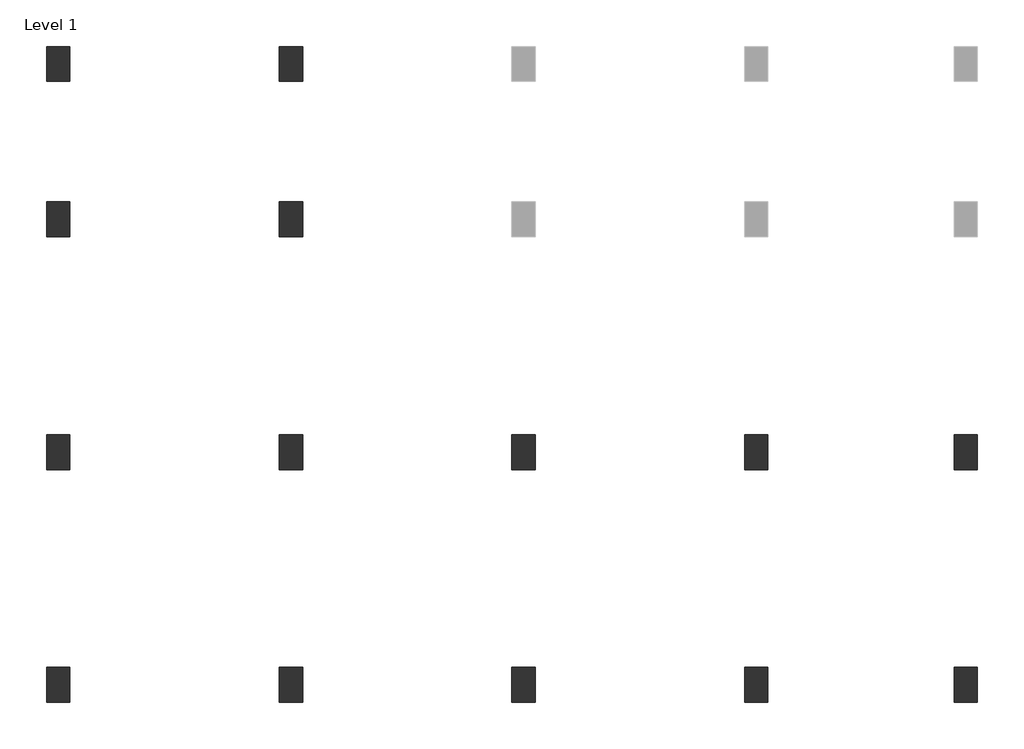
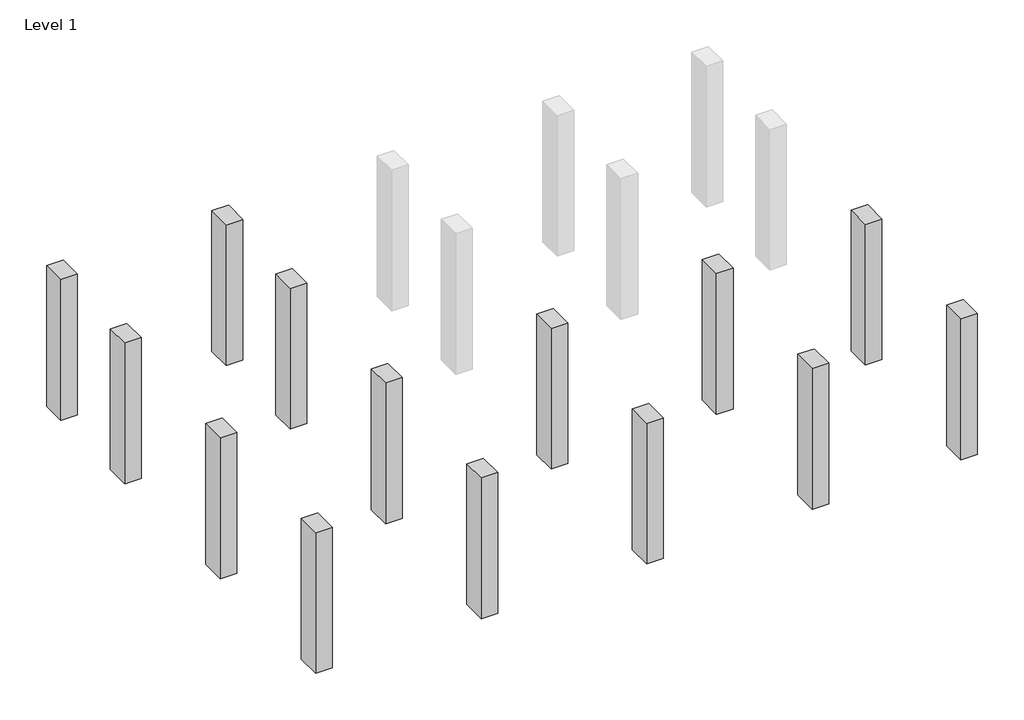
# One storey, part 1 of 2: 28 columns.
"""IFC4 building model written with IfcOpenShell, lengths in millimetres."""

from ifc_helpers import new_model, si_unit, frame, origin, place, context, project, spatial, polyline, outline, extrude, faceted_brep, element, save

model = new_model("IFC4")

# Units and contexts
model_context = context("Model", 3, world=origin())
ifc_project = project(units=[si_unit("LENGTHUNIT", "METRE", prefix="MILLI")], contexts=[model_context])

# Site, building, storey
site = spatial("IfcSite", under=ifc_project)
building = spatial("IfcBuilding", under=site)
storey = spatial("IfcBuildingStorey", under=building, Name="Level 1", Elevation=1219.2)

# Columns
placement = place(None, origin())
element("IfcColumn", 1, ObjectType="Concrete-Rectangular-Column : c1", at=placement, inside=storey, context=model_context, shape_type="SweptSolid", body=[
    extrude(outline(polyline([(-12327.4396417, 7215.6647757), (-12327.4396417, 7672.8647757), (-12022.6396417, 7672.8647757), (-12022.6396417, 7215.6647757), (-12327.4396417, 7215.6647757)])), frame((0.0, 0.0, 1219.2), z_axis=(0.0, 0.0, 1.0), x_axis=(1.0, 0.0, 0.0)), (0.0, 0.0, 1.0), 2743.2),
])
element("IfcColumn", 2, ObjectType="Concrete-Rectangular-Column : c1", at=placement, inside=storey, context=model_context, shape_type="SweptSolid", body=[
    extrude(outline(polyline([(-9279.4396417, 7215.6647757), (-9279.4396417, 7672.8647757), (-8974.6396417, 7672.8647757), (-8974.6396417, 7215.6647757), (-9279.4396417, 7215.6647757)])), frame((0.0, 0.0, 1219.2), z_axis=(0.0, 0.0, 1.0), x_axis=(1.0, 0.0, 0.0)), (0.0, 0.0, 1.0), 2743.2),
])
element("IfcColumn", 3, ObjectType="Concrete-Rectangular-Column : c1", at=placement, inside=storey, context=model_context, shape_type="SweptSolid", body=[
    extrude(outline(polyline([(-6231.4396417, 7215.6647757), (-6231.4396417, 7672.8647757), (-5926.6396417, 7672.8647757), (-5926.6396417, 7215.6647757), (-6231.4396417, 7215.6647757)])), frame((0.0, 0.0, 1219.2), z_axis=(0.0, 0.0, 1.0), x_axis=(1.0, 0.0, 0.0)), (0.0, 0.0, 1.0), 2743.2),
])
element("IfcColumn", 4, ObjectType="Concrete-Rectangular-Column : c1", at=placement, inside=storey, context=model_context, shape_type="SweptSolid", body=[
    extrude(outline(polyline([(-3183.4396417, 7215.6647757), (-3183.4396417, 7672.8647757), (-2878.6396417, 7672.8647757), (-2878.6396417, 7215.6647757), (-3183.4396417, 7215.6647757)])), frame((0.0, 0.0, 1219.2), z_axis=(0.0, 0.0, 1.0), x_axis=(1.0, 0.0, 0.0)), (0.0, 0.0, 1.0), 2743.2),
])
element("IfcColumn", 5, ObjectType="Concrete-Rectangular-Column : c1", at=placement, inside=storey, context=model_context, shape_type="SweptSolid", body=[
    extrude(outline(polyline([(-440.2396417, 7215.6647757), (-440.2396417, 7672.8647757), (-135.4396417, 7672.8647757), (-135.4396417, 7215.6647757), (-440.2396417, 7215.6647757)])), frame((0.0, 0.0, 1219.2), z_axis=(0.0, 0.0, 1.0), x_axis=(1.0, 0.0, 0.0)), (0.0, 0.0, 1.0), 2743.2),
])
element("IfcColumn", 6, ObjectType="Concrete-Rectangular-Column : c1", at=placement, inside=storey, context=model_context, shape_type="Brep", body=[
    faceted_brep([(-12327.4396417, 10263.6647757, 1219.2), (-12327.4396417, 10720.8647757, 1219.2), (-12022.6396417, 10720.8647757, 1219.2), (-12022.6396417, 10263.6647757, 1219.2), (-12327.4396417, 10263.6647757, 3962.4), (-12327.4396417, 10720.8647757, 3962.4), (-12327.4396417, 10720.8647757, 2743.2), (-12327.4396417, 10720.8647757, 2133.6), (-12327.4396417, 10263.6647757, 2133.6), (-12327.4396417, 10263.6647757, 2743.2), (-12022.6396417, 10720.8647757, 3962.4), (-12022.6396417, 10720.8647757, 2743.2), (-12022.6396417, 10720.8647757, 2133.6), (-12022.6396417, 10263.6647757, 3962.4), (-12022.6396417, 10263.6647757, 2743.2), (-12022.6396417, 10263.6647757, 2133.6)], [[[0, 1, 2, 3]], [[4, 5, 6, 7, 1, 0, 8, 9]], [[5, 10, 11, 12, 2, 1, 7, 6]], [[10, 13, 14, 15, 3, 2, 12, 11]], [[13, 4, 9, 8, 0, 3, 15, 14]], [[4, 13, 10, 5]]]),
])
element("IfcColumn", 7, ObjectType="Concrete-Rectangular-Column : c1", at=placement, inside=storey, context=model_context, shape_type="Brep", body=[
    faceted_brep([(-9279.4396417, 10263.6647757, 1219.2), (-9279.4396417, 10720.8647757, 1219.2), (-8974.6396417, 10720.8647757, 1219.2), (-8974.6396417, 10263.6647757, 1219.2), (-9279.4396417, 10263.6647757, 3962.4), (-9279.4396417, 10720.8647757, 3962.4), (-9279.4396417, 10720.8647757, 2743.2), (-9279.4396417, 10720.8647757, 2133.6), (-9279.4396417, 10263.6647757, 2133.6), (-9279.4396417, 10263.6647757, 2743.2), (-8974.6396417, 10720.8647757, 3962.4), (-8974.6396417, 10720.8647757, 2743.2), (-8974.6396417, 10720.8647757, 2133.6), (-8974.6396417, 10263.6647757, 3962.4), (-8974.6396417, 10263.6647757, 2743.2), (-8974.6396417, 10263.6647757, 2133.6)], [[[0, 1, 2, 3]], [[4, 5, 6, 7, 1, 0, 8, 9]], [[5, 10, 11, 12, 2, 1, 7, 6]], [[10, 13, 14, 15, 3, 2, 12, 11]], [[13, 4, 9, 8, 0, 3, 15, 14]], [[4, 13, 10, 5]]]),
])
element("IfcColumn", 8, ObjectType="Concrete-Rectangular-Column : c1", at=placement, inside=storey, context=model_context, shape_type="Brep", body=[
    faceted_brep([(-6231.4396417, 10263.6647757, 1219.2), (-6231.4396417, 10720.8647757, 1219.2), (-5926.6396417, 10720.8647757, 1219.2), (-5926.6396417, 10263.6647757, 1219.2), (-6231.4396417, 10263.6647757, 3962.4), (-6231.4396417, 10720.8647757, 3962.4), (-6231.4396417, 10720.8647757, 2743.2), (-6231.4396417, 10720.8647757, 2133.6), (-6231.4396417, 10263.6647757, 2133.6), (-6231.4396417, 10263.6647757, 2743.2), (-5926.6396417, 10720.8647757, 3962.4), (-5926.6396417, 10720.8647757, 2743.2), (-5926.6396417, 10720.8647757, 2133.6), (-5926.6396417, 10263.6647757, 3962.4), (-5926.6396417, 10263.6647757, 2743.2), (-5926.6396417, 10263.6647757, 2133.6)], [[[0, 1, 2, 3]], [[4, 5, 6, 7, 1, 0, 8, 9]], [[5, 10, 11, 12, 2, 1, 7, 6]], [[10, 13, 14, 15, 3, 2, 12, 11]], [[13, 4, 9, 8, 0, 3, 15, 14]], [[4, 13, 10, 5]]]),
])
element("IfcColumn", 9, ObjectType="Concrete-Rectangular-Column : c1", at=placement, inside=storey, context=model_context, shape_type="Brep", body=[
    faceted_brep([(-3183.4396417, 10263.6647757, 1219.2), (-3183.4396417, 10720.8647757, 1219.2), (-2878.6396417, 10720.8647757, 1219.2), (-2878.6396417, 10263.6647757, 1219.2), (-3183.4396417, 10263.6647757, 3962.4), (-3183.4396417, 10720.8647757, 3962.4), (-3183.4396417, 10720.8647757, 2743.2), (-3183.4396417, 10720.8647757, 2133.6), (-3183.4396417, 10263.6647757, 2133.6), (-3183.4396417, 10263.6647757, 2743.2), (-2878.6396417, 10720.8647757, 3962.4), (-2878.6396417, 10720.8647757, 2743.2), (-2878.6396417, 10720.8647757, 2133.6), (-2878.6396417, 10263.6647757, 3962.4), (-2878.6396417, 10263.6647757, 2743.2), (-2878.6396417, 10263.6647757, 2133.6)], [[[0, 1, 2, 3]], [[4, 5, 6, 7, 1, 0, 8, 9]], [[5, 10, 11, 12, 2, 1, 7, 6]], [[10, 13, 14, 15, 3, 2, 12, 11]], [[13, 4, 9, 8, 0, 3, 15, 14]], [[4, 13, 10, 5]]]),
])
element("IfcColumn", 10, ObjectType="Concrete-Rectangular-Column : c1", at=placement, inside=storey, context=model_context, shape_type="Brep", body=[
    faceted_brep([(-440.2396417, 10263.6647757, 1219.2), (-440.2396417, 10720.8647757, 1219.2), (-135.4396417, 10720.8647757, 1219.2), (-135.4396417, 10263.6647757, 1219.2), (-440.2396417, 10263.6647757, 3962.4), (-440.2396417, 10720.8647757, 3962.4), (-440.2396417, 10720.8647757, 2743.2), (-440.2396417, 10720.8647757, 2133.6), (-440.2396417, 10263.6647757, 2133.6), (-440.2396417, 10263.6647757, 2743.2), (-135.4396417, 10720.8647757, 3962.4), (-135.4396417, 10720.8647757, 2743.2), (-135.4396417, 10720.8647757, 2133.6), (-135.4396417, 10263.6647757, 3962.4), (-135.4396417, 10263.6647757, 2743.2), (-135.4396417, 10263.6647757, 2133.6)], [[[0, 1, 2, 3]], [[4, 5, 6, 7, 1, 0, 8, 9]], [[5, 10, 11, 12, 2, 1, 7, 6]], [[10, 13, 14, 15, 3, 2, 12, 11]], [[13, 4, 9, 8, 0, 3, 15, 14]], [[4, 13, 10, 5]]]),
])
element("IfcColumn", 11, ObjectType="Concrete-Rectangular-Column : c1", at=placement, inside=storey, context=model_context, shape_type="Brep", body=[
    faceted_brep([(-12327.4396417, 13311.6647757, 1219.2), (-12327.4396417, 13768.8647757, 1219.2), (-12022.6396417, 13768.8647757, 1219.2), (-12022.6396417, 13311.6647757, 1219.2), (-12327.4396417, 13311.6647757, 3962.4), (-12327.4396417, 13768.8647757, 3962.4), (-12327.4396417, 13768.8647757, 2743.2), (-12327.4396417, 13768.8647757, 2133.6), (-12327.4396417, 13311.6647757, 2133.6), (-12327.4396417, 13311.6647757, 2743.2), (-12022.6396417, 13768.8647757, 3962.4), (-12022.6396417, 13768.8647757, 2743.2), (-12022.6396417, 13768.8647757, 2133.6), (-12022.6396417, 13311.6647757, 3962.4), (-12022.6396417, 13311.6647757, 2743.2), (-12022.6396417, 13311.6647757, 2133.6)], [[[0, 1, 2, 3]], [[4, 5, 6, 7, 1, 0, 8, 9]], [[5, 10, 11, 12, 2, 1, 7, 6]], [[10, 13, 14, 15, 3, 2, 12, 11]], [[13, 4, 9, 8, 0, 3, 15, 14]], [[4, 13, 10, 5]]]),
])
element("IfcColumn", 12, ObjectType="Concrete-Rectangular-Column : c1", at=placement, inside=storey, context=model_context, shape_type="Brep", body=[
    faceted_brep([(-9279.4396417, 13311.6647757, 1219.2), (-9279.4396417, 13768.8647757, 1219.2), (-8974.6396417, 13768.8647757, 1219.2), (-8974.6396417, 13311.6647757, 1219.2), (-9279.4396417, 13311.6647757, 3962.4), (-9279.4396417, 13768.8647757, 3962.4), (-9279.4396417, 13768.8647757, 2743.2), (-9279.4396417, 13768.8647757, 2133.6), (-9279.4396417, 13311.6647757, 2133.6), (-9279.4396417, 13311.6647757, 2743.2), (-8974.6396417, 13768.8647757, 3962.4), (-8974.6396417, 13768.8647757, 2743.2), (-8974.6396417, 13768.8647757, 2133.6), (-8974.6396417, 13311.6647757, 3962.4), (-8974.6396417, 13311.6647757, 2743.2), (-8974.6396417, 13311.6647757, 2133.6)], [[[0, 1, 2, 3]], [[4, 5, 6, 7, 1, 0, 8, 9]], [[5, 10, 11, 12, 2, 1, 7, 6]], [[10, 13, 14, 15, 3, 2, 12, 11]], [[13, 4, 9, 8, 0, 3, 15, 14]], [[4, 13, 10, 5]]]),
])
element("IfcColumn", 13, ObjectType="Concrete-Rectangular-Column : c1", at=placement, inside=storey, context=model_context, shape_type="Brep", body=[
    faceted_brep([(-12327.4396417, 15346.9119241, 1219.2), (-12327.4396417, 15804.1119241, 1219.2), (-12022.6396417, 15804.1119241, 1219.2), (-12022.6396417, 15346.9119241, 1219.2), (-12327.4396417, 15346.9119241, 3962.4), (-12327.4396417, 15804.1119241, 3962.4), (-12327.4396417, 15804.1119241, 2743.2), (-12327.4396417, 15804.1119241, 2133.6), (-12327.4396417, 15346.9119241, 2133.6), (-12327.4396417, 15346.9119241, 2743.2), (-12022.6396417, 15804.1119241, 3962.4), (-12022.6396417, 15804.1119241, 2743.2), (-12022.6396417, 15804.1119241, 2133.6), (-12022.6396417, 15346.9119241, 3962.4), (-12022.6396417, 15346.9119241, 2743.2), (-12022.6396417, 15346.9119241, 2133.6)], [[[0, 1, 2, 3]], [[4, 5, 6, 7, 1, 0, 8, 9]], [[5, 10, 11, 12, 2, 1, 7, 6]], [[10, 13, 14, 15, 3, 2, 12, 11]], [[13, 4, 9, 8, 0, 3, 15, 14]], [[4, 13, 10, 5]]]),
])
element("IfcColumn", 14, ObjectType="Concrete-Rectangular-Column : c1", at=placement, inside=storey, context=model_context, shape_type="Brep", body=[
    faceted_brep([(-9279.4396417, 15346.9119241, 1219.2), (-9279.4396417, 15804.1119241, 1219.2), (-8974.6396417, 15804.1119241, 1219.2), (-8974.6396417, 15346.9119241, 1219.2), (-9279.4396417, 15346.9119241, 3962.4), (-9279.4396417, 15804.1119241, 3962.4), (-9279.4396417, 15804.1119241, 2743.2), (-9279.4396417, 15804.1119241, 2133.6), (-9279.4396417, 15346.9119241, 2133.6), (-9279.4396417, 15346.9119241, 2743.2), (-8974.6396417, 15804.1119241, 3962.4), (-8974.6396417, 15804.1119241, 2743.2), (-8974.6396417, 15804.1119241, 2133.6), (-8974.6396417, 15346.9119241, 3962.4), (-8974.6396417, 15346.9119241, 2743.2), (-8974.6396417, 15346.9119241, 2133.6)], [[[0, 1, 2, 3]], [[4, 5, 6, 7, 1, 0, 8, 9]], [[5, 10, 11, 12, 2, 1, 7, 6]], [[10, 13, 14, 15, 3, 2, 12, 11]], [[13, 4, 9, 8, 0, 3, 15, 14]], [[4, 13, 10, 5]]]),
])
element("IfcColumn", 15, ObjectType="Concrete-Rectangular-Column : c1", at=placement, inside=storey, context=model_context, shape_type="Brep", body=[
    faceted_brep([(-12327.4396417, 7215.6647757, 1219.2), (-12327.4396417, 7672.8647757, 1219.2), (-12022.6396417, 7672.8647757, 1219.2), (-12022.6396417, 7215.6647757, 1219.2), (-12327.4396417, 7215.6647757, 3962.4), (-12327.4396417, 7672.8647757, 3962.4), (-12327.4396417, 7672.8647757, 2743.2), (-12327.4396417, 7672.8647757, 2133.6), (-12022.6396417, 7672.8647757, 3962.4), (-12022.6396417, 7672.8647757, 2743.2), (-12022.6396417, 7672.8647757, 2133.6), (-12022.6396417, 7215.6647757, 3962.4)], [[[0, 1, 2, 3]], [[4, 5, 6, 7, 1, 0]], [[5, 8, 9, 10, 2, 1, 7, 6]], [[8, 11, 3, 2, 10, 9]], [[11, 4, 0, 3]], [[4, 11, 8, 5]]]),
])
element("IfcColumn", 16, ObjectType="Concrete-Rectangular-Column : c1", at=placement, inside=storey, context=model_context, shape_type="Brep", body=[
    faceted_brep([(-9279.4396417, 7215.6647757, 1219.2), (-9279.4396417, 7672.8647757, 1219.2), (-8974.6396417, 7672.8647757, 1219.2), (-8974.6396417, 7215.6647757, 1219.2), (-9279.4396417, 7215.6647757, 3962.4), (-9279.4396417, 7672.8647757, 3962.4), (-9279.4396417, 7672.8647757, 2743.2), (-9279.4396417, 7672.8647757, 2133.6), (-8974.6396417, 7672.8647757, 3962.4), (-8974.6396417, 7672.8647757, 2743.2), (-8974.6396417, 7672.8647757, 2133.6), (-8974.6396417, 7215.6647757, 3962.4)], [[[0, 1, 2, 3]], [[4, 5, 6, 7, 1, 0]], [[5, 8, 9, 10, 2, 1, 7, 6]], [[8, 11, 3, 2, 10, 9]], [[11, 4, 0, 3]], [[4, 11, 8, 5]]]),
])
element("IfcColumn", 17, ObjectType="Concrete-Rectangular-Column : c1", at=placement, inside=storey, context=model_context, shape_type="Brep", body=[
    faceted_brep([(-6231.4396417, 7215.6647757, 1219.2), (-6231.4396417, 7672.8647757, 1219.2), (-5926.6396417, 7672.8647757, 1219.2), (-5926.6396417, 7215.6647757, 1219.2), (-6231.4396417, 7215.6647757, 3962.4), (-6231.4396417, 7672.8647757, 3962.4), (-6231.4396417, 7672.8647757, 2743.2), (-6231.4396417, 7672.8647757, 2133.6), (-5926.6396417, 7672.8647757, 3962.4), (-5926.6396417, 7672.8647757, 2743.2), (-5926.6396417, 7672.8647757, 2133.6), (-5926.6396417, 7215.6647757, 3962.4)], [[[0, 1, 2, 3]], [[4, 5, 6, 7, 1, 0]], [[5, 8, 9, 10, 2, 1, 7, 6]], [[8, 11, 3, 2, 10, 9]], [[11, 4, 0, 3]], [[4, 11, 8, 5]]]),
])
element("IfcColumn", 18, ObjectType="Concrete-Rectangular-Column : c1", at=placement, inside=storey, context=model_context, shape_type="Brep", body=[
    faceted_brep([(-3183.4396417, 7215.6647757, 1219.2), (-3183.4396417, 7672.8647757, 1219.2), (-2878.6396417, 7672.8647757, 1219.2), (-2878.6396417, 7215.6647757, 1219.2), (-3183.4396417, 7215.6647757, 3962.4), (-3183.4396417, 7672.8647757, 3962.4), (-3183.4396417, 7672.8647757, 2743.2), (-3183.4396417, 7672.8647757, 2133.6), (-2878.6396417, 7672.8647757, 3962.4), (-2878.6396417, 7672.8647757, 2743.2), (-2878.6396417, 7672.8647757, 2133.6), (-2878.6396417, 7215.6647757, 3962.4)], [[[0, 1, 2, 3]], [[4, 5, 6, 7, 1, 0]], [[5, 8, 9, 10, 2, 1, 7, 6]], [[8, 11, 3, 2, 10, 9]], [[11, 4, 0, 3]], [[4, 11, 8, 5]]]),
])
element("IfcColumn", 19, ObjectType="Concrete-Rectangular-Column : c1", at=placement, inside=storey, context=model_context, shape_type="Brep", body=[
    faceted_brep([(-440.2396417, 7215.6647757, 1219.2), (-440.2396417, 7672.8647757, 1219.2), (-135.4396417, 7672.8647757, 1219.2), (-135.4396417, 7215.6647757, 1219.2), (-440.2396417, 7215.6647757, 3962.4), (-440.2396417, 7672.8647757, 3962.4), (-440.2396417, 7672.8647757, 2743.2), (-440.2396417, 7672.8647757, 2133.6), (-135.4396417, 7672.8647757, 3962.4), (-135.4396417, 7672.8647757, 2743.2), (-135.4396417, 7672.8647757, 2133.6), (-135.4396417, 7215.6647757, 3962.4)], [[[0, 1, 2, 3]], [[4, 5, 6, 7, 1, 0]], [[5, 8, 9, 10, 2, 1, 7, 6]], [[8, 11, 3, 2, 10, 9]], [[11, 4, 0, 3]], [[4, 11, 8, 5]]]),
])
element("IfcColumn", 20, ObjectType="Concrete-Rectangular-Column : c1", at=placement, inside=storey, context=model_context, shape_type="Brep", body=[
    faceted_brep([(-12327.4396417, 10263.6647757, 1219.2), (-12327.4396417, 10720.8647757, 1219.2), (-12022.6396417, 10720.8647757, 1219.2), (-12022.6396417, 10263.6647757, 1219.2), (-12327.4396417, 10263.6647757, 3962.4), (-12327.4396417, 10720.8647757, 3962.4), (-12327.4396417, 10720.8647757, 2743.2), (-12327.4396417, 10720.8647757, 2133.6), (-12327.4396417, 10263.6647757, 2133.6), (-12327.4396417, 10263.6647757, 2743.2), (-12022.6396417, 10720.8647757, 3962.4), (-12022.6396417, 10720.8647757, 2743.2), (-12022.6396417, 10720.8647757, 2133.6), (-12022.6396417, 10263.6647757, 3962.4), (-12022.6396417, 10263.6647757, 2743.2), (-12022.6396417, 10263.6647757, 2133.6)], [[[0, 1, 2, 3]], [[4, 5, 6, 7, 1, 0, 8, 9]], [[5, 10, 11, 12, 2, 1, 7, 6]], [[10, 13, 14, 15, 3, 2, 12, 11]], [[13, 4, 9, 8, 0, 3, 15, 14]], [[4, 13, 10, 5]]]),
])
element("IfcColumn", 21, ObjectType="Concrete-Rectangular-Column : c1", at=placement, inside=storey, context=model_context, shape_type="Brep", body=[
    faceted_brep([(-9279.4396417, 10263.6647757, 1219.2), (-9279.4396417, 10720.8647757, 1219.2), (-8974.6396417, 10720.8647757, 1219.2), (-8974.6396417, 10263.6647757, 1219.2), (-9279.4396417, 10263.6647757, 3962.4), (-9279.4396417, 10720.8647757, 3962.4), (-9279.4396417, 10720.8647757, 2743.2), (-9279.4396417, 10720.8647757, 2133.6), (-9279.4396417, 10263.6647757, 2133.6), (-9279.4396417, 10263.6647757, 2743.2), (-8974.6396417, 10720.8647757, 3962.4), (-8974.6396417, 10720.8647757, 2743.2), (-8974.6396417, 10720.8647757, 2133.6), (-8974.6396417, 10263.6647757, 3962.4), (-8974.6396417, 10263.6647757, 2743.2), (-8974.6396417, 10263.6647757, 2133.6)], [[[0, 1, 2, 3]], [[4, 5, 6, 7, 1, 0, 8, 9]], [[5, 10, 11, 12, 2, 1, 7, 6]], [[10, 13, 14, 15, 3, 2, 12, 11]], [[13, 4, 9, 8, 0, 3, 15, 14]], [[4, 13, 10, 5]]]),
])
element("IfcColumn", 22, ObjectType="Concrete-Rectangular-Column : c1", at=placement, inside=storey, context=model_context, shape_type="Brep", body=[
    faceted_brep([(-6231.4396417, 10263.6647757, 1219.2), (-6231.4396417, 10720.8647757, 1219.2), (-5926.6396417, 10720.8647757, 1219.2), (-5926.6396417, 10263.6647757, 1219.2), (-6231.4396417, 10263.6647757, 3962.4), (-6231.4396417, 10720.8647757, 3962.4), (-6231.4396417, 10720.8647757, 2743.2), (-6231.4396417, 10720.8647757, 2133.6), (-6231.4396417, 10263.6647757, 2133.6), (-6231.4396417, 10263.6647757, 2743.2), (-5926.6396417, 10720.8647757, 3962.4), (-5926.6396417, 10720.8647757, 2743.2), (-5926.6396417, 10720.8647757, 2133.6), (-5926.6396417, 10263.6647757, 3962.4), (-5926.6396417, 10263.6647757, 2743.2), (-5926.6396417, 10263.6647757, 2133.6)], [[[0, 1, 2, 3]], [[4, 5, 6, 7, 1, 0, 8, 9]], [[5, 10, 11, 12, 2, 1, 7, 6]], [[10, 13, 14, 15, 3, 2, 12, 11]], [[13, 4, 9, 8, 0, 3, 15, 14]], [[4, 13, 10, 5]]]),
])
element("IfcColumn", 23, ObjectType="Concrete-Rectangular-Column : c1", at=placement, inside=storey, context=model_context, shape_type="Brep", body=[
    faceted_brep([(-3183.4396417, 10263.6647757, 1219.2), (-3183.4396417, 10720.8647757, 1219.2), (-2878.6396417, 10720.8647757, 1219.2), (-2878.6396417, 10263.6647757, 1219.2), (-3183.4396417, 10263.6647757, 3962.4), (-3183.4396417, 10720.8647757, 3962.4), (-3183.4396417, 10720.8647757, 2743.2), (-3183.4396417, 10720.8647757, 2133.6), (-3183.4396417, 10263.6647757, 2133.6), (-3183.4396417, 10263.6647757, 2743.2), (-2878.6396417, 10720.8647757, 3962.4), (-2878.6396417, 10720.8647757, 2743.2), (-2878.6396417, 10720.8647757, 2133.6), (-2878.6396417, 10263.6647757, 3962.4), (-2878.6396417, 10263.6647757, 2743.2), (-2878.6396417, 10263.6647757, 2133.6)], [[[0, 1, 2, 3]], [[4, 5, 6, 7, 1, 0, 8, 9]], [[5, 10, 11, 12, 2, 1, 7, 6]], [[10, 13, 14, 15, 3, 2, 12, 11]], [[13, 4, 9, 8, 0, 3, 15, 14]], [[4, 13, 10, 5]]]),
])
element("IfcColumn", 24, ObjectType="Concrete-Rectangular-Column : c1", at=placement, inside=storey, context=model_context, shape_type="Brep", body=[
    faceted_brep([(-440.2396417, 10263.6647757, 1219.2), (-440.2396417, 10720.8647757, 1219.2), (-135.4396417, 10720.8647757, 1219.2), (-135.4396417, 10263.6647757, 1219.2), (-440.2396417, 10263.6647757, 3962.4), (-440.2396417, 10720.8647757, 3962.4), (-440.2396417, 10720.8647757, 2743.2), (-440.2396417, 10720.8647757, 2133.6), (-440.2396417, 10263.6647757, 2133.6), (-440.2396417, 10263.6647757, 2743.2), (-135.4396417, 10720.8647757, 3962.4), (-135.4396417, 10720.8647757, 2743.2), (-135.4396417, 10720.8647757, 2133.6), (-135.4396417, 10263.6647757, 3962.4), (-135.4396417, 10263.6647757, 2743.2), (-135.4396417, 10263.6647757, 2133.6)], [[[0, 1, 2, 3]], [[4, 5, 6, 7, 1, 0, 8, 9]], [[5, 10, 11, 12, 2, 1, 7, 6]], [[10, 13, 14, 15, 3, 2, 12, 11]], [[13, 4, 9, 8, 0, 3, 15, 14]], [[4, 13, 10, 5]]]),
])
element("IfcColumn", 25, ObjectType="Concrete-Rectangular-Column : c1", at=placement, inside=storey, context=model_context, shape_type="Brep", body=[
    faceted_brep([(-12327.4396417, 13311.6647757, 1219.2), (-12327.4396417, 13768.8647757, 1219.2), (-12022.6396417, 13768.8647757, 1219.2), (-12022.6396417, 13311.6647757, 1219.2), (-12327.4396417, 13311.6647757, 3962.4), (-12327.4396417, 13768.8647757, 3962.4), (-12327.4396417, 13768.8647757, 2743.2), (-12327.4396417, 13768.8647757, 2133.6), (-12327.4396417, 13311.6647757, 2133.6), (-12327.4396417, 13311.6647757, 2743.2), (-12022.6396417, 13768.8647757, 3962.4), (-12022.6396417, 13768.8647757, 2743.2), (-12022.6396417, 13768.8647757, 2133.6), (-12022.6396417, 13311.6647757, 3962.4), (-12022.6396417, 13311.6647757, 2743.2), (-12022.6396417, 13311.6647757, 2133.6)], [[[0, 1, 2, 3]], [[4, 5, 6, 7, 1, 0, 8, 9]], [[5, 10, 11, 12, 2, 1, 7, 6]], [[10, 13, 14, 15, 3, 2, 12, 11]], [[13, 4, 9, 8, 0, 3, 15, 14]], [[4, 13, 10, 5]]]),
])
element("IfcColumn", 26, ObjectType="Concrete-Rectangular-Column : c1", at=placement, inside=storey, context=model_context, shape_type="Brep", body=[
    faceted_brep([(-9279.4396417, 13311.6647757, 1219.2), (-9279.4396417, 13768.8647757, 1219.2), (-8974.6396417, 13768.8647757, 1219.2), (-8974.6396417, 13311.6647757, 1219.2), (-9279.4396417, 13311.6647757, 3962.4), (-9279.4396417, 13768.8647757, 3962.4), (-9279.4396417, 13768.8647757, 2743.2), (-9279.4396417, 13768.8647757, 2133.6), (-9279.4396417, 13311.6647757, 2133.6), (-9279.4396417, 13311.6647757, 2743.2), (-8974.6396417, 13768.8647757, 3962.4), (-8974.6396417, 13768.8647757, 2743.2), (-8974.6396417, 13768.8647757, 2133.6), (-8974.6396417, 13311.6647757, 3962.4), (-8974.6396417, 13311.6647757, 2743.2), (-8974.6396417, 13311.6647757, 2133.6)], [[[0, 1, 2, 3]], [[4, 5, 6, 7, 1, 0, 8, 9]], [[5, 10, 11, 12, 2, 1, 7, 6]], [[10, 13, 14, 15, 3, 2, 12, 11]], [[13, 4, 9, 8, 0, 3, 15, 14]], [[4, 13, 10, 5]]]),
])
element("IfcColumn", 27, ObjectType="Concrete-Rectangular-Column : c1", at=placement, inside=storey, context=model_context, shape_type="Brep", body=[
    faceted_brep([(-12327.4396417, 15346.9119241, 1219.2), (-12327.4396417, 15804.1119241, 1219.2), (-12022.6396417, 15804.1119241, 1219.2), (-12022.6396417, 15346.9119241, 1219.2), (-12327.4396417, 15346.9119241, 3962.4), (-12327.4396417, 15804.1119241, 3962.4), (-12327.4396417, 15804.1119241, 2743.2), (-12327.4396417, 15804.1119241, 2133.6), (-12327.4396417, 15346.9119241, 2133.6), (-12327.4396417, 15346.9119241, 2743.2), (-12022.6396417, 15804.1119241, 3962.4), (-12022.6396417, 15804.1119241, 2743.2), (-12022.6396417, 15804.1119241, 2133.6), (-12022.6396417, 15346.9119241, 3962.4), (-12022.6396417, 15346.9119241, 2743.2), (-12022.6396417, 15346.9119241, 2133.6)], [[[0, 1, 2, 3]], [[4, 5, 6, 7, 1, 0, 8, 9]], [[5, 10, 11, 12, 2, 1, 7, 6]], [[10, 13, 14, 15, 3, 2, 12, 11]], [[13, 4, 9, 8, 0, 3, 15, 14]], [[4, 13, 10, 5]]]),
])
element("IfcColumn", 28, ObjectType="Concrete-Rectangular-Column : c1", at=placement, inside=storey, context=model_context, shape_type="Brep", body=[
    faceted_brep([(-9279.4396417, 15346.9119241, 1219.2), (-9279.4396417, 15804.1119241, 1219.2), (-8974.6396417, 15804.1119241, 1219.2), (-8974.6396417, 15346.9119241, 1219.2), (-9279.4396417, 15346.9119241, 3962.4), (-9279.4396417, 15804.1119241, 3962.4), (-9279.4396417, 15804.1119241, 2743.2), (-9279.4396417, 15804.1119241, 2133.6), (-9279.4396417, 15346.9119241, 2133.6), (-9279.4396417, 15346.9119241, 2743.2), (-8974.6396417, 15804.1119241, 3962.4), (-8974.6396417, 15804.1119241, 2743.2), (-8974.6396417, 15804.1119241, 2133.6), (-8974.6396417, 15346.9119241, 3962.4), (-8974.6396417, 15346.9119241, 2743.2), (-8974.6396417, 15346.9119241, 2133.6)], [[[0, 1, 2, 3]], [[4, 5, 6, 7, 1, 0, 8, 9]], [[5, 10, 11, 12, 2, 1, 7, 6]], [[10, 13, 14, 15, 3, 2, 12, 11]], [[13, 4, 9, 8, 0, 3, 15, 14]], [[4, 13, 10, 5]]]),
])

save(model, "model.ifc")

# Revit data of these elements
# Type "Concrete-Rectangular-Column : c1"
#   Assembly Code = "B10"
#   b = 1' - 0"
#   h = 1' - 6"
#   Structural Material [instance default] = Concrete, Cast-in-Place gray
# Elements 1, 2, 3, 4, 5, 6, 7, 8, 9, 10, 11, 12, 13, 14, 15, 16, 17, 18, 19, 20, 21, 22, 23, 24, 25, 26, 27, 28 (IfcColumn, "Concrete-Rectangular-Column : c1")
#   Comments = ""
#   Structural Material = Concrete, Cast-in-Place gray
#   Phase Created = New Construction
#   Materials on its faces: "Concrete, Cast-in-Place gray"
# Materials
#   "Concrete, Cast-in-Place gray": class "Concrete", colour RGB 192 192 192, transparency 0, Description = "Cast-in-place concrete", Cost = 0
